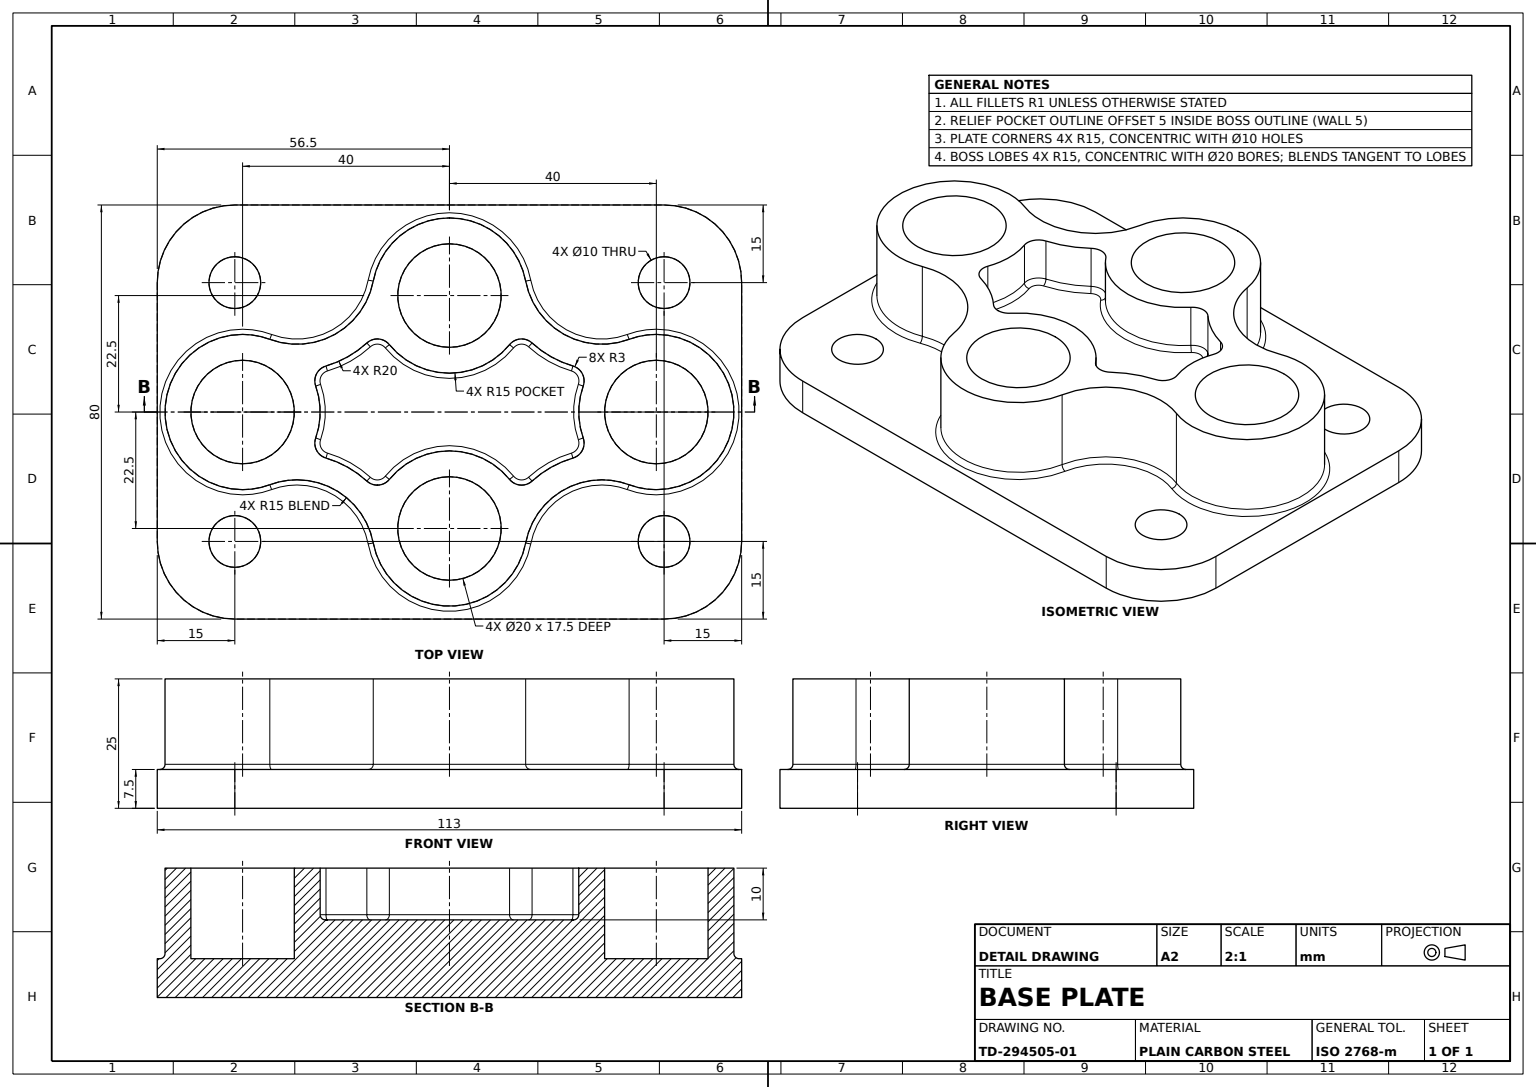
SolidWorks part; units mm, degrees
material "Plain Carbon Steel"
ref_plane "Front Plane" through (0, 0, 0) normal (0, 0, 1) x (1, 0, 0)
ref_plane "Top Plane" through (0, 0, 0) normal (0, 1, 0) x (1, 0, 0)
ref_plane "Right Plane" through (0, 0, 0) normal (1, 0, 0) x (0, 0, -1)
sketch "Base Plate Sketch" plane through (0, 0, 0) normal (0, 1, 0) x (1, 0, 0)
  line L1 (-56.5, -40) -> (56.5, -40)
  line L2 (-56.5, -40) -> (-56.5, 40)
  line L3 (-56.5, 40) -> (56.5, 40)
  line L4 (56.5, -40) -> (56.5, 40)
  line L5 (-56.5, -40) -> (56.5, 40) construction
  line L6 (-56.5, 40) -> (56.5, -40) construction
  point P0 (0, 0)
  dimension "D1" = 113
  dimension "D2" = 80
extrude "Base Plate 113x80x7.5" add sketch "Base Plate Sketch" along normal blind 7.5
fillet "Plate Corner Fillets R15" radius 15 4 edges at (56.5, 3.75, -40) (56.5, 3.75, 40) (-56.5, 3.75, 40) (-56.5, 3.75, -40)
sketch "Mounting Holes Sketch" plane through (0, 7.5, 0) normal (0, 1, 0) x (1, 0, 0)
  circle A0 centre (-41.5, 25) radius 5
  circle A1 centre (41.5, 25) radius 5
  circle A2 centre (-41.5, -25) radius 5
  circle A3 centre (41.5, -25) radius 5
  dimension "D1" = 10
  dimension "D2" = 10
  dimension "D3" = 10
  dimension "D4" = 10
extrude "Corner Mounting Holes 4x" cut sketch "Mounting Holes Sketch" against normal blind 7.5
sketch "Bore Boss Cluster Sketch" plane through (0, 7.5, 0) normal (0, 1, 0) x (1, 0, 0)
  line L0 (41.5, 40) -> (-41.5, 40) construction
  line L2 (56.5, -25) -> (56.5, 25) construction
  arc A0 (-34.737, 14.0464) -> (-34.737, -14.0464) centre (-40, 0) ccw
  circle A4 centre (-40, 0) radius 10
  circle A5 centre (0, 22.5) radius 10
  circle A6 centre (40, 0) radius 10
  circle A7 centre (0, -22.5) radius 10
  arc A8 (-34.737, 14.0464) -> (-14.737, 25.2964) centre (-29.4741, 28.0928) ccw
  arc A9 (14.737, 25.2964) -> (34.737, 14.0464) centre (29.4741, 28.0928) ccw
  arc A10 (-34.737, -14.0464) -> (-14.737, -25.2964) centre (-29.4741, -28.0928) cw
  arc A11 (14.737, -25.2964) -> (34.737, -14.0464) centre (29.4741, -28.0928) cw
  arc A18 (14.737, 25.2964) -> (-14.737, 25.2964) centre (0, 22.5) ccw
  arc A21 (34.737, -14.0464) -> (34.737, 14.0464) centre (40, 0) ccw
  arc A22 (-14.737, -25.2964) -> (14.737, -25.2964) centre (0, -22.5) ccw
  point P29 (-29.4741, 28.0928)
  point P30 (-36.4914, 9.3643)
  point P31 (-9.8247, 24.3643)
  point P32 (29.4741, 28.0928)
  point P33 (9.8247, 24.3643)
  point P34 (36.4914, 9.3643)
  point P35 (-29.4741, -28.0928)
  point P36 (-36.4914, -9.3643)
  point P37 (-9.8247, -24.3643)
  point P38 (29.4741, -28.0928)
  point P39 (9.8247, -24.3643)
  point P40 (36.4914, -9.3643)
  dimension "D2" = 40
  dimension "D7" = 56.5
  dimension "D8" = 56.5
  dimension "D13" = 20
  dimension "D10" = 15
  dimension "D11" = 15
  dimension "D3" = 40
  dimension "D4" = 40
  dimension "D5" = 22.5
  dimension "D6" = 40
  dimension "D9" = 22.5
extrude "Bore Boss Cluster" add sketch "Bore Boss Cluster Sketch" along normal blind 17.5
sketch "Bores and Relief Pocket Sketch" plane through (0, 25, 0) normal (0, 1, 0) x (1, 0, 0)
  arc A0 (-23.874, -8.8928) -> (-25.8616, -5.0107) centre (-23.034, -6.0128) cw
  arc A1 (-15.9738, -13.3366) -> (-11.624, -13.0194) centre (-13.9488, -11.1232) ccw
  circle A2 centre (-40, 0) radius 15
  arc A3 (-25.8616, -5.0107) -> (-25.8616, 5.0107) centre (-40, 0) ccw
  arc A4 (15.9738, -13.3366) -> (11.624, -13.0194) centre (13.9488, -11.1232) cw
  arc A5 (-36.4914, 9.3643) -> (-9.8247, 24.3643) centre (-29.4741, 28.0928) ccw
  arc A6 (-23.874, 8.8928) -> (-15.9738, 13.3366) centre (-29.4741, 28.0928) ccw
  circle A7 centre (0, 22.5) radius 15
  arc A8 (9.8247, 24.3643) -> (36.4914, 9.3643) centre (29.4741, 28.0928) ccw
  arc A9 (15.9738, 13.3366) -> (23.874, 8.8928) centre (29.4741, 28.0928) ccw
  arc A10 (-11.624, 13.0194) -> (11.624, 13.0194) centre (0, 22.5) ccw
  arc A11 (36.4914, -9.3643) -> (9.8247, -24.3643) centre (29.4741, -28.0928) ccw
  arc A12 (23.874, -8.8928) -> (15.9738, -13.3366) centre (29.4741, -28.0928) ccw
  arc A13 (23.874, -8.8928) -> (25.8616, -5.0107) centre (23.034, -6.0128) ccw
  circle A14 centre (40, 0) radius 15
  arc A15 (25.8616, 5.0107) -> (25.8616, -5.0107) centre (40, 0) ccw
  arc A16 (25.8616, 5.0107) -> (23.874, 8.8928) centre (23.034, 6.0128) ccw
  circle A17 centre (0, -22.5) radius 15
  arc A18 (11.624, -13.0194) -> (-11.624, -13.0194) centre (0, -22.5) ccw
  arc A19 (15.9738, 13.3366) -> (11.624, 13.0194) centre (13.9488, 11.1232) ccw
  arc A20 (-15.9738, 13.3366) -> (-11.624, 13.0194) centre (-13.9488, 11.1232) cw
  arc A21 (-25.8616, 5.0107) -> (-23.874, 8.8928) centre (-23.034, 6.0128) cw
  arc A22 (-9.8247, -24.3643) -> (-36.4914, -9.3643) centre (-29.4741, -28.0928) ccw
  arc A23 (-15.9738, -13.3366) -> (-23.874, -8.8928) centre (-29.4741, -28.0928) ccw
  dimension "D9" = 3
  dimension "D1" = 5
  dimension "D2" = 5
  dimension "D3" = 5
  dimension "D4" = 5
  dimension "D5" = 5
  dimension "D6" = 5
  dimension "D7" = 5
  dimension "D8" = 5
extrude "Bores and Relief Pocket" cut sketch "Bores and Relief Pocket Sketch" against normal blind 10
fillet "Boss Root Fillet R1" radius 1 8 edges at (-22.1201, 7.5, 15.0192) (-55, 7.5, 0) (-22.1201, 7.5, -15.0192) (0, 7.5, -37.5) (22.1201, 7.5, -15.0192) (55, 7.5, 0) (22.1201, 7.5, 15.0192) (0, 7.5, 37.5)
fillet "Bore and Pocket Edge Fillet R1" radius 1 16 edges at (13.7305, 15, -14.1153) (19.6688, 15, -10.6613) (25.7043, 15, -7.38) (25, 15, 0) (25.7043, 15, 7.38) (19.6688, 15, 10.6613) (13.7305, 15, 14.1153) (0, 15, 7.5) (-13.7305, 15, 14.1153) (-19.6688, 15, 10.6613) (-25.7043, 15, 7.38) (-25, 15, 0) (-25.7043, 15, -7.38) (-19.6688, 15, -10.6613) (-13.7305, 15, -14.1153) (0, 15, -7.5)
